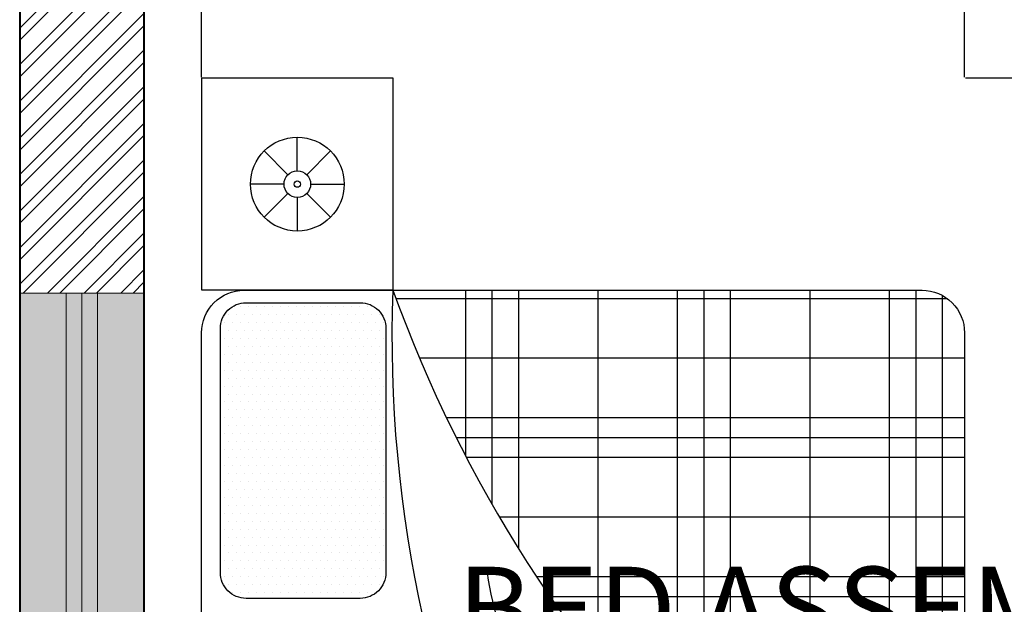
# Model space of a CAD drawing. Units: inches. Extents: x 528 to 2520, y -151 to 1354.
# Tile 5 of 41: x 587 to 658, y 1189 to 1232. Entities that reach past the tile are written whole.
import ezdxf

# ---------------------------------------------------------------- set-up
doc = ezdxf.new("R2010")
doc.units = ezdxf.units.IN
doc.header["$MEASUREMENT"] = 0
for name, color, linetype, lineweight in [('A-ANNO-DIMS', 2, 'Continuous', 18), ('A-FURN', 8, 'Continuous', 18), ('A-WALL-PATT', 6, 'Continuous', 13), ('walls', 7, 'Continuous', 40), ('WINDOWS', 2, 'Continuous', 20)]:
    doc.layers.add(name, color=color, linetype=linetype, lineweight=lineweight)
doc.layers.add('A-GLAZ-PATT', color=152, linetype='Continuous', lineweight=13, true_color=0x2776bb)
doc.layers.add('BLOCK', color=6, linetype='Continuous')
doc.styles.get("Standard").update_dxf_attribs({"font": 'arial.ttf'})
doc.dimstyles.get("Standard").update_dxf_attribs({"dimtxt": 6, "dimasz": 2, "dimexe": 0.18, "dimexo": 0.0625, "dimgap": 0.09, "dimtad": 0, "dimtih": 1, "dimtoh": 1, "dimdec": 1, "dimzin": 0, "dimdsep": 46, "dimlunit": 3, "dimtxsty": 'Standard', "dimblk": 'ARCHTICK', "dimcen": 0.09, "dimadec": 0, "dimazin": 0, "dimtfac": 1, "dimtdec": 1, "dimtofl": 0, "dimtmove": 0, "dimatfit": 3, "dimfxl": 1, "dimtolj": 1, "dimtzin": 0, "dimarcsym": 0})

# ---------------------------------------------------------------- blocks, each defined once
blk = doc.blocks.new('*X15')
at = {"color": 0}
for p, q in [((276.598, 451.25), (280.51, 451.25)), ((275.455, 450.625), (280.51, 450.625)), ((274.411, 450), (280.51, 450)), ((265.51, 448.125), (267.634, 448.125)), ((271.723, 448.125), (280.51, 448.125)), ((265.51, 446.25), (268.465, 446.25)), ((269.519, 446.25), (280.51, 446.25)), ((265.51, 445.625), (268.531, 445.625)), ((268.866, 445.625), (280.51, 445.625)), ((265.51, 445), (280.51, 445)), ((265.51, 443.125), (280.51, 443.125)), ((265.51, 441.25), (280.51, 441.25)), ((265.51, 440.625), (280.51, 440.625)), ((265.634, 440), (280.386, 440))]:
    blk.add_line(p, q, dxfattribs=at)
blk = doc.blocks.new('*X16')
at = {"color": 0}
for p, q in [((280.312, 439.886), (280.312, 452.896)), ((278.906, 439.482), (278.906, 452.338)), ((277.5, 439.482), (277.5, 451.702)), ((277.031, 439.482), (277.031, 451.471)), ((276.562, 439.482), (276.562, 451.231)), ((275.156, 439.482), (275.156, 450.451)), ((265.781, 439.797), (265.781, 449.511)), ((273.75, 439.482), (273.75, 449.576)), ((266.25, 439.517), (266.25, 449.296)), ((273.281, 439.482), (273.281, 449.261)), ((272.812, 439.482), (272.812, 448.934)), ((267.656, 439.482), (267.656, 448.095)), ((271.406, 439.482), (271.406, 447.876)), ((270, 439.482), (270, 446.689)), ((269.531, 439.482), (269.531, 446.262)), ((269.062, 439.482), (269.062, 445.817))]:
    blk.add_line(p, q, dxfattribs=at)
blk = doc.blocks.new('*X17')
at = {"color": 0}
for p, q in [((273.9375, 457.03125), (273.9375, 457.03125)), ((274.3125, 457.03125), (274.3125, 457.03125)), ((274.6875, 457.03125), (274.6875, 457.03125)), ((275.0625, 457.03125), (275.0625, 457.03125)), ((275.4375, 457.03125), (275.4375, 457.03125)), ((275.8125, 457.03125), (275.8125, 457.03125)), ((276.1875, 457.03125), (276.1875, 457.03125)), ((276.5625, 457.03125), (276.5625, 457.03125)), ((276.9375, 457.03125), (276.9375, 457.03125)), ((277.3125, 457.03125), (277.3125, 457.03125)), ((277.6875, 457.03125), (277.6875, 457.03125)), ((278.0625, 457.03125), (278.0625, 457.03125)), ((278.4375, 457.03125), (278.4375, 457.03125)), ((278.8125, 457.03125), (278.8125, 457.03125)), ((279.1875, 457.03125), (279.1875, 457.03125)), ((279.5625, 457.03125), (279.5625, 457.03125)), ((273.375, 456.75), (273.375, 456.75)), ((273.5625, 456.84375), (273.5625, 456.84375)), ((273.75, 456.9375), (273.75, 456.9375)), ((273.75, 456.75), (273.75, 456.75)), ((273.9375, 456.84375), (273.9375, 456.84375)), ((274.125, 456.9375), (274.125, 456.9375)), ((274.125, 456.75), (274.125, 456.75)), ((274.3125, 456.84375), (274.3125, 456.84375)), ((274.5, 456.9375), (274.5, 456.9375)), ((274.5, 456.75), (274.5, 456.75)), ((274.6875, 456.84375), (274.6875, 456.84375)), ((274.875, 456.9375), (274.875, 456.9375)), ((274.875, 456.75), (274.875, 456.75)), ((275.0625, 456.84375), (275.0625, 456.84375)), ((275.25, 456.9375), (275.25, 456.9375)), ((275.25, 456.75), (275.25, 456.75)), ((275.4375, 456.84375), (275.4375, 456.84375)), ((275.625, 456.9375), (275.625, 456.9375)), ((275.625, 456.75), (275.625, 456.75)), ((275.8125, 456.84375), (275.8125, 456.84375)), ((276, 456.9375), (276, 456.9375)), ((276, 456.75), (276, 456.75)), ((276.1875, 456.84375), (276.1875, 456.84375)), ((276.375, 456.9375), (276.375, 456.9375)), ((276.375, 456.75), (276.375, 456.75)), ((276.5625, 456.84375), (276.5625, 456.84375)), ((276.75, 456.9375), (276.75, 456.9375)), ((276.75, 456.75), (276.75, 456.75)), ((276.9375, 456.84375), (276.9375, 456.84375)), ((277.125, 456.9375), (277.125, 456.9375)), ((277.125, 456.75), (277.125, 456.75)), ((277.3125, 456.84375), (277.3125, 456.84375)), ((277.5, 456.9375), (277.5, 456.9375)), ((277.5, 456.75), (277.5, 456.75)), ((277.6875, 456.84375), (277.6875, 456.84375)), ((277.875, 456.9375), (277.875, 456.9375)), ((277.875, 456.75), (277.875, 456.75)), ((278.0625, 456.84375), (278.0625, 456.84375)), ((278.25, 456.9375), (278.25, 456.9375)), ((278.25, 456.75), (278.25, 456.75)), ((278.4375, 456.84375), (278.4375, 456.84375)), ((278.625, 456.9375), (278.625, 456.9375)), ((278.625, 456.75), (278.625, 456.75)), ((278.8125, 456.84375), (278.8125, 456.84375)), ((279, 456.9375), (279, 456.9375)), ((279, 456.75), (279, 456.75)), ((279.1875, 456.84375), (279.1875, 456.84375)), ((279.375, 456.9375), (279.375, 456.9375)), ((279.375, 456.75), (279.375, 456.75)), ((279.5625, 456.84375), (279.5625, 456.84375)), ((279.75, 456.9375), (279.75, 456.9375)), ((279.75, 456.75), (279.75, 456.75)), ((279.9375, 456.84375), (279.9375, 456.84375)), ((280.125, 456.75), (280.125, 456.75)), ((273.375, 456.5625), (273.375, 456.5625)), ((273.5625, 456.65625), (273.5625, 456.65625)), ((273.75, 456.5625), (273.75, 456.5625)), ((273.9375, 456.65625), (273.9375, 456.65625)), ((274.125, 456.5625), (274.125, 456.5625)), ((274.3125, 456.65625), (274.3125, 456.65625)), ((274.5, 456.5625), (274.5, 456.5625)), ((274.6875, 456.65625), (274.6875, 456.65625)), ((274.875, 456.5625), (274.875, 456.5625)), ((275.0625, 456.65625), (275.0625, 456.65625)), ((275.25, 456.5625), (275.25, 456.5625)), ((275.4375, 456.65625), (275.4375, 456.65625)), ((275.625, 456.5625), (275.625, 456.5625)), ((275.8125, 456.65625), (275.8125, 456.65625)), ((276, 456.5625), (276, 456.5625)), ((276.1875, 456.65625), (276.1875, 456.65625)), ((276.375, 456.5625), (276.375, 456.5625)), ((276.5625, 456.65625), (276.5625, 456.65625)), ((276.75, 456.5625), (276.75, 456.5625)), ((276.9375, 456.65625), (276.9375, 456.65625)), ((277.125, 456.5625), (277.125, 456.5625)), ((277.3125, 456.65625), (277.3125, 456.65625)), ((277.5, 456.5625), (277.5, 456.5625)), ((277.6875, 456.65625), (277.6875, 456.65625)), ((277.875, 456.5625), (277.875, 456.5625)), ((278.0625, 456.65625), (278.0625, 456.65625)), ((278.25, 456.5625), (278.25, 456.5625)), ((278.4375, 456.65625), (278.4375, 456.65625)), ((278.625, 456.5625), (278.625, 456.5625)), ((278.8125, 456.65625), (278.8125, 456.65625)), ((279, 456.5625), (279, 456.5625)), ((279.1875, 456.65625), (279.1875, 456.65625)), ((279.375, 456.5625), (279.375, 456.5625)), ((279.5625, 456.65625), (279.5625, 456.65625)), ((279.75, 456.5625), (279.75, 456.5625)), ((279.9375, 456.65625), (279.9375, 456.65625)), ((280.125, 456.5625), (280.125, 456.5625)), ((273.375, 456.375), (273.375, 456.375)), ((273.5625, 456.46875), (273.5625, 456.46875)), ((273.5625, 456.28125), (273.5625, 456.28125)), ((273.75, 456.375), (273.75, 456.375)), ((273.9375, 456.46875), (273.9375, 456.46875)), ((273.9375, 456.28125), (273.9375, 456.28125)), ((274.125, 456.375), (274.125, 456.375)), ((274.3125, 456.46875), (274.3125, 456.46875)), ((274.3125, 456.28125), (274.3125, 456.28125)), ((274.5, 456.375), (274.5, 456.375)), ((274.6875, 456.46875), (274.6875, 456.46875)), ((274.6875, 456.28125), (274.6875, 456.28125)), ((274.875, 456.375), (274.875, 456.375)), ((275.0625, 456.46875), (275.0625, 456.46875)), ((275.0625, 456.28125), (275.0625, 456.28125)), ((275.25, 456.375), (275.25, 456.375)), ((275.4375, 456.46875), (275.4375, 456.46875)), ((275.4375, 456.28125), (275.4375, 456.28125)), ((275.625, 456.375), (275.625, 456.375)), ((275.8125, 456.46875), (275.8125, 456.46875)), ((275.8125, 456.28125), (275.8125, 456.28125)), ((276, 456.375), (276, 456.375)), ((276.1875, 456.46875), (276.1875, 456.46875)), ((276.1875, 456.28125), (276.1875, 456.28125)), ((276.375, 456.375), (276.375, 456.375)), ((276.5625, 456.46875), (276.5625, 456.46875)), ((276.5625, 456.28125), (276.5625, 456.28125)), ((276.75, 456.375), (276.75, 456.375)), ((276.9375, 456.46875), (276.9375, 456.46875)), ((276.9375, 456.28125), (276.9375, 456.28125)), ((277.125, 456.375), (277.125, 456.375)), ((277.3125, 456.46875), (277.3125, 456.46875)), ((277.3125, 456.28125), (277.3125, 456.28125)), ((277.5, 456.375), (277.5, 456.375)), ((277.6875, 456.46875), (277.6875, 456.46875)), ((277.6875, 456.28125), (277.6875, 456.28125)), ((277.875, 456.375), (277.875, 456.375)), ((278.0625, 456.46875), (278.0625, 456.46875)), ((278.0625, 456.28125), (278.0625, 456.28125)), ((278.25, 456.375), (278.25, 456.375)), ((278.4375, 456.46875), (278.4375, 456.46875)), ((278.4375, 456.28125), (278.4375, 456.28125)), ((278.625, 456.375), (278.625, 456.375)), ((278.8125, 456.46875), (278.8125, 456.46875)), ((278.8125, 456.28125), (278.8125, 456.28125)), ((279, 456.375), (279, 456.375)), ((279.1875, 456.46875), (279.1875, 456.46875)), ((279.1875, 456.28125), (279.1875, 456.28125)), ((279.375, 456.375), (279.375, 456.375)), ((279.5625, 456.46875), (279.5625, 456.46875)), ((279.5625, 456.28125), (279.5625, 456.28125)), ((279.75, 456.375), (279.75, 456.375)), ((279.9375, 456.46875), (279.9375, 456.46875)), ((279.9375, 456.28125), (279.9375, 456.28125)), ((280.125, 456.375), (280.125, 456.375)), ((273.375, 456.1875), (273.375, 456.1875)), ((273.5625, 456.09375), (273.5625, 456.09375)), ((273.75, 456.1875), (273.75, 456.1875)), ((273.9375, 456.09375), (273.9375, 456.09375)), ((274.125, 456.1875), (274.125, 456.1875)), ((274.3125, 456.09375), (274.3125, 456.09375)), ((274.5, 456.1875), (274.5, 456.1875)), ((274.6875, 456.09375), (274.6875, 456.09375)), ((274.875, 456.1875), (274.875, 456.1875)), ((275.0625, 456.09375), (275.0625, 456.09375)), ((275.25, 456.1875), (275.25, 456.1875)), ((275.4375, 456.09375), (275.4375, 456.09375)), ((275.625, 456.1875), (275.625, 456.1875)), ((275.8125, 456.09375), (275.8125, 456.09375)), ((276, 456.1875), (276, 456.1875)), ((276.1875, 456.09375), (276.1875, 456.09375)), ((276.375, 456.1875), (276.375, 456.1875)), ((276.5625, 456.09375), (276.5625, 456.09375)), ((276.75, 456.1875), (276.75, 456.1875)), ((276.9375, 456.09375), (276.9375, 456.09375)), ((277.125, 456.1875), (277.125, 456.1875)), ((277.3125, 456.09375), (277.3125, 456.09375)), ((277.5, 456.1875), (277.5, 456.1875)), ((277.6875, 456.09375), (277.6875, 456.09375)), ((277.875, 456.1875), (277.875, 456.1875)), ((278.0625, 456.09375), (278.0625, 456.09375)), ((278.25, 456.1875), (278.25, 456.1875)), ((278.4375, 456.09375), (278.4375, 456.09375)), ((278.625, 456.1875), (278.625, 456.1875)), ((278.8125, 456.09375), (278.8125, 456.09375)), ((279, 456.1875), (279, 456.1875)), ((279.1875, 456.09375), (279.1875, 456.09375)), ((279.375, 456.1875), (279.375, 456.1875)), ((279.5625, 456.09375), (279.5625, 456.09375)), ((279.75, 456.1875), (279.75, 456.1875)), ((279.9375, 456.09375), (279.9375, 456.09375)), ((280.125, 456.1875), (280.125, 456.1875)), ((273.375, 456), (273.375, 456)), ((273.375, 455.8125), (273.375, 455.8125)), ((273.5625, 455.90625), (273.5625, 455.90625)), ((273.75, 456), (273.75, 456)), ((273.75, 455.8125), (273.75, 455.8125)), ((273.9375, 455.90625), (273.9375, 455.90625)), ((274.125, 456), (274.125, 456)), ((274.125, 455.8125), (274.125, 455.8125)), ((274.3125, 455.90625), (274.3125, 455.90625)), ((274.5, 456), (274.5, 456)), ((274.5, 455.8125), (274.5, 455.8125)), ((274.6875, 455.90625), (274.6875, 455.90625)), ((274.875, 456), (274.875, 456)), ((274.875, 455.8125), (274.875, 455.8125)), ((275.0625, 455.90625), (275.0625, 455.90625)), ((275.25, 456), (275.25, 456)), ((275.25, 455.8125), (275.25, 455.8125)), ((275.4375, 455.90625), (275.4375, 455.90625)), ((275.625, 456), (275.625, 456)), ((275.625, 455.8125), (275.625, 455.8125)), ((275.8125, 455.90625), (275.8125, 455.90625)), ((276, 456), (276, 456)), ((276, 455.8125), (276, 455.8125)), ((276.1875, 455.90625), (276.1875, 455.90625)), ((276.375, 456), (276.375, 456)), ((276.375, 455.8125), (276.375, 455.8125)), ((276.5625, 455.90625), (276.5625, 455.90625)), ((276.75, 456), (276.75, 456)), ((276.75, 455.8125), (276.75, 455.8125)), ((276.9375, 455.90625), (276.9375, 455.90625)), ((277.125, 456), (277.125, 456)), ((277.125, 455.8125), (277.125, 455.8125)), ((277.3125, 455.90625), (277.3125, 455.90625)), ((277.5, 456), (277.5, 456)), ((277.5, 455.8125), (277.5, 455.8125)), ((277.6875, 455.90625), (277.6875, 455.90625)), ((277.875, 456), (277.875, 456)), ((277.875, 455.8125), (277.875, 455.8125)), ((278.0625, 455.90625), (278.0625, 455.90625)), ((278.25, 456), (278.25, 456)), ((278.25, 455.8125), (278.25, 455.8125)), ((278.4375, 455.90625), (278.4375, 455.90625)), ((278.625, 456), (278.625, 456)), ((278.625, 455.8125), (278.625, 455.8125)), ((278.8125, 455.90625), (278.8125, 455.90625)), ((279, 456), (279, 456)), ((279, 455.8125), (279, 455.8125)), ((279.1875, 455.90625), (279.1875, 455.90625)), ((279.375, 456), (279.375, 456)), ((279.375, 455.8125), (279.375, 455.8125)), ((279.5625, 455.90625), (279.5625, 455.90625)), ((279.75, 456), (279.75, 456)), ((279.75, 455.8125), (279.75, 455.8125)), ((279.9375, 455.90625), (279.9375, 455.90625)), ((280.125, 456), (280.125, 456)), ((280.125, 455.8125), (280.125, 455.8125)), ((273.375, 455.625), (273.375, 455.625)), ((273.5625, 455.71875), (273.5625, 455.71875)), ((273.75, 455.625), (273.75, 455.625)), ((273.9375, 455.71875), (273.9375, 455.71875)), ((274.125, 455.625), (274.125, 455.625)), ((274.3125, 455.71875), (274.3125, 455.71875)), ((274.5, 455.625), (274.5, 455.625)), ((274.6875, 455.71875), (274.6875, 455.71875)), ((274.875, 455.625), (274.875, 455.625)), ((275.0625, 455.71875), (275.0625, 455.71875)), ((275.25, 455.625), (275.25, 455.625)), ((275.4375, 455.71875), (275.4375, 455.71875)), ((275.625, 455.625), (275.625, 455.625)), ((275.8125, 455.71875), (275.8125, 455.71875)), ((276, 455.625), (276, 455.625)), ((276.1875, 455.71875), (276.1875, 455.71875)), ((276.375, 455.625), (276.375, 455.625)), ((276.5625, 455.71875), (276.5625, 455.71875)), ((276.75, 455.625), (276.75, 455.625)), ((276.9375, 455.71875), (276.9375, 455.71875)), ((277.125, 455.625), (277.125, 455.625)), ((277.3125, 455.71875), (277.3125, 455.71875)), ((277.5, 455.625), (277.5, 455.625)), ((277.6875, 455.71875), (277.6875, 455.71875)), ((277.875, 455.625), (277.875, 455.625)), ((278.0625, 455.71875), (278.0625, 455.71875)), ((278.25, 455.625), (278.25, 455.625)), ((278.4375, 455.71875), (278.4375, 455.71875)), ((278.625, 455.625), (278.625, 455.625)), ((278.8125, 455.71875), (278.8125, 455.71875)), ((279, 455.625), (279, 455.625)), ((279.1875, 455.71875), (279.1875, 455.71875)), ((279.375, 455.625), (279.375, 455.625)), ((279.5625, 455.71875), (279.5625, 455.71875)), ((279.75, 455.625), (279.75, 455.625)), ((279.9375, 455.71875), (279.9375, 455.71875)), ((280.125, 455.625), (280.125, 455.625)), ((273.375, 455.4375), (273.375, 455.4375)), ((273.5625, 455.53125), (273.5625, 455.53125)), ((273.5625, 455.34375), (273.5625, 455.34375)), ((273.75, 455.4375), (273.75, 455.4375)), ((273.9375, 455.53125), (273.9375, 455.53125)), ((273.9375, 455.34375), (273.9375, 455.34375)), ((274.125, 455.4375), (274.125, 455.4375)), ((274.3125, 455.53125), (274.3125, 455.53125)), ((274.3125, 455.34375), (274.3125, 455.34375)), ((274.5, 455.4375), (274.5, 455.4375)), ((274.6875, 455.53125), (274.6875, 455.53125)), ((274.6875, 455.34375), (274.6875, 455.34375)), ((274.875, 455.4375), (274.875, 455.4375)), ((275.0625, 455.53125), (275.0625, 455.53125)), ((275.0625, 455.34375), (275.0625, 455.34375)), ((275.25, 455.4375), (275.25, 455.4375)), ((275.4375, 455.53125), (275.4375, 455.53125)), ((275.4375, 455.34375), (275.4375, 455.34375)), ((275.625, 455.4375), (275.625, 455.4375)), ((275.8125, 455.53125), (275.8125, 455.53125)), ((275.8125, 455.34375), (275.8125, 455.34375)), ((276, 455.4375), (276, 455.4375)), ((276.1875, 455.53125), (276.1875, 455.53125)), ((276.1875, 455.34375), (276.1875, 455.34375)), ((276.375, 455.4375), (276.375, 455.4375)), ((276.5625, 455.53125), (276.5625, 455.53125)), ((276.5625, 455.34375), (276.5625, 455.34375)), ((276.75, 455.4375), (276.75, 455.4375)), ((276.9375, 455.53125), (276.9375, 455.53125)), ((276.9375, 455.34375), (276.9375, 455.34375)), ((277.125, 455.4375), (277.125, 455.4375)), ((277.3125, 455.53125), (277.3125, 455.53125)), ((277.3125, 455.34375), (277.3125, 455.34375)), ((277.5, 455.4375), (277.5, 455.4375)), ((277.6875, 455.53125), (277.6875, 455.53125)), ((277.6875, 455.34375), (277.6875, 455.34375)), ((277.875, 455.4375), (277.875, 455.4375)), ((278.0625, 455.53125), (278.0625, 455.53125)), ((278.0625, 455.34375), (278.0625, 455.34375)), ((278.25, 455.4375), (278.25, 455.4375)), ((278.4375, 455.53125), (278.4375, 455.53125)), ((278.4375, 455.34375), (278.4375, 455.34375)), ((278.625, 455.4375), (278.625, 455.4375)), ((278.8125, 455.53125), (278.8125, 455.53125)), ((278.8125, 455.34375), (278.8125, 455.34375)), ((279, 455.4375), (279, 455.4375)), ((279.1875, 455.53125), (279.1875, 455.53125)), ((279.1875, 455.34375), (279.1875, 455.34375)), ((279.375, 455.4375), (279.375, 455.4375)), ((279.5625, 455.53125), (279.5625, 455.53125)), ((279.5625, 455.34375), (279.5625, 455.34375)), ((279.75, 455.4375), (279.75, 455.4375)), ((279.9375, 455.53125), (279.9375, 455.53125)), ((279.9375, 455.34375), (279.9375, 455.34375)), ((280.125, 455.4375), (280.125, 455.4375)), ((273.375, 455.25), (273.375, 455.25)), ((273.5625, 455.15625), (273.5625, 455.15625)), ((273.75, 455.25), (273.75, 455.25)), ((273.9375, 455.15625), (273.9375, 455.15625)), ((274.125, 455.25), (274.125, 455.25)), ((274.3125, 455.15625), (274.3125, 455.15625)), ((274.5, 455.25), (274.5, 455.25)), ((274.6875, 455.15625), (274.6875, 455.15625)), ((274.875, 455.25), (274.875, 455.25)), ((275.0625, 455.15625), (275.0625, 455.15625)), ((275.25, 455.25), (275.25, 455.25)), ((275.4375, 455.15625), (275.4375, 455.15625)), ((275.625, 455.25), (275.625, 455.25)), ((275.8125, 455.15625), (275.8125, 455.15625)), ((276, 455.25), (276, 455.25)), ((276.1875, 455.15625), (276.1875, 455.15625)), ((276.375, 455.25), (276.375, 455.25)), ((276.5625, 455.15625), (276.5625, 455.15625)), ((276.75, 455.25), (276.75, 455.25)), ((276.9375, 455.15625), (276.9375, 455.15625)), ((277.125, 455.25), (277.125, 455.25)), ((277.3125, 455.15625), (277.3125, 455.15625)), ((277.5, 455.25), (277.5, 455.25)), ((277.6875, 455.15625), (277.6875, 455.15625)), ((277.875, 455.25), (277.875, 455.25)), ((278.0625, 455.15625), (278.0625, 455.15625)), ((278.25, 455.25), (278.25, 455.25)), ((278.4375, 455.15625), (278.4375, 455.15625)), ((278.625, 455.25), (278.625, 455.25)), ((278.8125, 455.15625), (278.8125, 455.15625)), ((279, 455.25), (279, 455.25)), ((279.1875, 455.15625), (279.1875, 455.15625)), ((279.375, 455.25), (279.375, 455.25)), ((279.5625, 455.15625), (279.5625, 455.15625)), ((279.75, 455.25), (279.75, 455.25)), ((279.9375, 455.15625), (279.9375, 455.15625)), ((280.125, 455.25), (280.125, 455.25)), ((273.375, 455.0625), (273.375, 455.0625)), ((273.375, 454.875), (273.375, 454.875)), ((273.5625, 454.96875), (273.5625, 454.96875)), ((273.75, 455.0625), (273.75, 455.0625)), ((273.75, 454.875), (273.75, 454.875)), ((273.9375, 454.96875), (273.9375, 454.96875)), ((274.125, 455.0625), (274.125, 455.0625)), ((274.125, 454.875), (274.125, 454.875)), ((274.3125, 454.96875), (274.3125, 454.96875)), ((274.5, 455.0625), (274.5, 455.0625)), ((274.5, 454.875), (274.5, 454.875)), ((274.6875, 454.96875), (274.6875, 454.96875)), ((274.875, 455.0625), (274.875, 455.0625)), ((274.875, 454.875), (274.875, 454.875)), ((275.0625, 454.96875), (275.0625, 454.96875)), ((275.25, 455.0625), (275.25, 455.0625)), ((275.25, 454.875), (275.25, 454.875)), ((275.4375, 454.96875), (275.4375, 454.96875)), ((275.625, 455.0625), (275.625, 455.0625)), ((275.625, 454.875), (275.625, 454.875)), ((275.8125, 454.96875), (275.8125, 454.96875)), ((276, 455.0625), (276, 455.0625)), ((276, 454.875), (276, 454.875)), ((276.1875, 454.96875), (276.1875, 454.96875)), ((276.375, 455.0625), (276.375, 455.0625)), ((276.375, 454.875), (276.375, 454.875)), ((276.5625, 454.96875), (276.5625, 454.96875)), ((276.75, 455.0625), (276.75, 455.0625)), ((276.75, 454.875), (276.75, 454.875)), ((276.9375, 454.96875), (276.9375, 454.96875)), ((277.125, 455.0625), (277.125, 455.0625)), ((277.125, 454.875), (277.125, 454.875)), ((277.3125, 454.96875), (277.3125, 454.96875)), ((277.5, 455.0625), (277.5, 455.0625)), ((277.5, 454.875), (277.5, 454.875)), ((277.6875, 454.96875), (277.6875, 454.96875)), ((277.875, 455.0625), (277.875, 455.0625)), ((277.875, 454.875), (277.875, 454.875)), ((278.0625, 454.96875), (278.0625, 454.96875)), ((278.25, 455.0625), (278.25, 455.0625)), ((278.25, 454.875), (278.25, 454.875)), ((278.4375, 454.96875), (278.4375, 454.96875)), ((278.625, 455.0625), (278.625, 455.0625)), ((278.625, 454.875), (278.625, 454.875)), ((278.8125, 454.96875), (278.8125, 454.96875)), ((279, 455.0625), (279, 455.0625)), ((279, 454.875), (279, 454.875)), ((279.1875, 454.96875), (279.1875, 454.96875)), ((279.375, 455.0625), (279.375, 455.0625)), ((279.375, 454.875), (279.375, 454.875)), ((279.5625, 454.96875), (279.5625, 454.96875)), ((279.75, 455.0625), (279.75, 455.0625)), ((279.75, 454.875), (279.75, 454.875)), ((279.9375, 454.96875), (279.9375, 454.96875)), ((280.125, 455.0625), (280.125, 455.0625)), ((280.125, 454.875), (280.125, 454.875)), ((273.375, 454.6875), (273.375, 454.6875)), ((273.5625, 454.78125), (273.5625, 454.78125)), ((273.75, 454.6875), (273.75, 454.6875)), ((273.9375, 454.78125), (273.9375, 454.78125)), ((274.125, 454.6875), (274.125, 454.6875)), ((274.3125, 454.78125), (274.3125, 454.78125)), ((274.5, 454.6875), (274.5, 454.6875)), ((274.6875, 454.78125), (274.6875, 454.78125)), ((274.875, 454.6875), (274.875, 454.6875)), ((275.0625, 454.78125), (275.0625, 454.78125)), ((275.25, 454.6875), (275.25, 454.6875)), ((275.4375, 454.78125), (275.4375, 454.78125)), ((275.625, 454.6875), (275.625, 454.6875)), ((275.8125, 454.78125), (275.8125, 454.78125)), ((276, 454.6875), (276, 454.6875)), ((276.1875, 454.78125), (276.1875, 454.78125)), ((276.375, 454.6875), (276.375, 454.6875)), ((276.5625, 454.78125), (276.5625, 454.78125)), ((276.75, 454.6875), (276.75, 454.6875)), ((276.9375, 454.78125), (276.9375, 454.78125)), ((277.125, 454.6875), (277.125, 454.6875)), ((277.3125, 454.78125), (277.3125, 454.78125)), ((277.5, 454.6875), (277.5, 454.6875)), ((277.6875, 454.78125), (277.6875, 454.78125)), ((277.875, 454.6875), (277.875, 454.6875)), ((278.0625, 454.78125), (278.0625, 454.78125)), ((278.25, 454.6875), (278.25, 454.6875)), ((278.4375, 454.78125), (278.4375, 454.78125)), ((278.625, 454.6875), (278.625, 454.6875)), ((278.8125, 454.78125), (278.8125, 454.78125)), ((279, 454.6875), (279, 454.6875)), ((279.1875, 454.78125), (279.1875, 454.78125)), ((279.375, 454.6875), (279.375, 454.6875)), ((279.5625, 454.78125), (279.5625, 454.78125)), ((279.75, 454.6875), (279.75, 454.6875)), ((279.9375, 454.78125), (279.9375, 454.78125)), ((280.125, 454.6875), (280.125, 454.6875)), ((273.375, 454.5), (273.375, 454.5)), ((273.5625, 454.59375), (273.5625, 454.59375)), ((273.5625, 454.40625), (273.5625, 454.40625)), ((273.75, 454.5), (273.75, 454.5)), ((273.9375, 454.59375), (273.9375, 454.59375)), ((273.9375, 454.40625), (273.9375, 454.40625)), ((274.125, 454.5), (274.125, 454.5)), ((274.3125, 454.59375), (274.3125, 454.59375)), ((274.3125, 454.40625), (274.3125, 454.40625)), ((274.5, 454.5), (274.5, 454.5)), ((274.6875, 454.59375), (274.6875, 454.59375)), ((274.6875, 454.40625), (274.6875, 454.40625)), ((274.875, 454.5), (274.875, 454.5)), ((275.0625, 454.59375), (275.0625, 454.59375)), ((275.0625, 454.40625), (275.0625, 454.40625)), ((275.25, 454.5), (275.25, 454.5)), ((275.4375, 454.59375), (275.4375, 454.59375)), ((275.4375, 454.40625), (275.4375, 454.40625)), ((275.625, 454.5), (275.625, 454.5)), ((275.8125, 454.59375), (275.8125, 454.59375)), ((275.8125, 454.40625), (275.8125, 454.40625)), ((276, 454.5), (276, 454.5)), ((276.1875, 454.59375), (276.1875, 454.59375)), ((276.1875, 454.40625), (276.1875, 454.40625)), ((276.375, 454.5), (276.375, 454.5)), ((276.5625, 454.59375), (276.5625, 454.59375)), ((276.5625, 454.40625), (276.5625, 454.40625)), ((276.75, 454.5), (276.75, 454.5)), ((276.9375, 454.59375), (276.9375, 454.59375)), ((276.9375, 454.40625), (276.9375, 454.40625)), ((277.125, 454.5), (277.125, 454.5)), ((277.3125, 454.59375), (277.3125, 454.59375)), ((277.3125, 454.40625), (277.3125, 454.40625)), ((277.5, 454.5), (277.5, 454.5)), ((277.6875, 454.59375), (277.6875, 454.59375)), ((277.6875, 454.40625), (277.6875, 454.40625)), ((277.875, 454.5), (277.875, 454.5)), ((278.0625, 454.59375), (278.0625, 454.59375)), ((278.0625, 454.40625), (278.0625, 454.40625)), ((278.25, 454.5), (278.25, 454.5)), ((278.4375, 454.59375), (278.4375, 454.59375)), ((278.4375, 454.40625), (278.4375, 454.40625)), ((278.625, 454.5), (278.625, 454.5)), ((278.8125, 454.59375), (278.8125, 454.59375)), ((278.8125, 454.40625), (278.8125, 454.40625)), ((279, 454.5), (279, 454.5)), ((279.1875, 454.59375), (279.1875, 454.59375)), ((279.1875, 454.40625), (279.1875, 454.40625)), ((279.375, 454.5), (279.375, 454.5)), ((279.5625, 454.59375), (279.5625, 454.59375)), ((279.5625, 454.40625), (279.5625, 454.40625)), ((279.75, 454.5), (279.75, 454.5)), ((279.9375, 454.59375), (279.9375, 454.59375)), ((279.9375, 454.40625), (279.9375, 454.40625)), ((280.125, 454.5), (280.125, 454.5)), ((273.375, 454.3125), (273.375, 454.3125)), ((273.5625, 454.21875), (273.5625, 454.21875)), ((273.75, 454.3125), (273.75, 454.3125)), ((273.9375, 454.21875), (273.9375, 454.21875)), ((274.125, 454.3125), (274.125, 454.3125)), ((274.3125, 454.21875), (274.3125, 454.21875)), ((274.5, 454.3125), (274.5, 454.3125)), ((274.6875, 454.21875), (274.6875, 454.21875)), ((274.875, 454.3125), (274.875, 454.3125)), ((275.0625, 454.21875), (275.0625, 454.21875)), ((275.25, 454.3125), (275.25, 454.3125)), ((275.4375, 454.21875), (275.4375, 454.21875)), ((275.625, 454.3125), (275.625, 454.3125)), ((275.8125, 454.21875), (275.8125, 454.21875)), ((276, 454.3125), (276, 454.3125)), ((276.1875, 454.21875), (276.1875, 454.21875)), ((276.375, 454.3125), (276.375, 454.3125)), ((276.5625, 454.21875), (276.5625, 454.21875)), ((276.75, 454.3125), (276.75, 454.3125)), ((276.9375, 454.21875), (276.9375, 454.21875)), ((277.125, 454.3125), (277.125, 454.3125)), ((277.3125, 454.21875), (277.3125, 454.21875)), ((277.5, 454.3125), (277.5, 454.3125)), ((277.6875, 454.21875), (277.6875, 454.21875)), ((277.875, 454.3125), (277.875, 454.3125)), ((278.0625, 454.21875), (278.0625, 454.21875)), ((278.25, 454.3125), (278.25, 454.3125)), ((278.4375, 454.21875), (278.4375, 454.21875)), ((278.625, 454.3125), (278.625, 454.3125)), ((278.8125, 454.21875), (278.8125, 454.21875)), ((279, 454.3125), (279, 454.3125)), ((279.1875, 454.21875), (279.1875, 454.21875)), ((279.375, 454.3125), (279.375, 454.3125)), ((279.5625, 454.21875), (279.5625, 454.21875)), ((279.75, 454.3125), (279.75, 454.3125)), ((279.9375, 454.21875), (279.9375, 454.21875)), ((280.125, 454.3125), (280.125, 454.3125)), ((273.375, 454.125), (273.375, 454.125)), ((273.375, 453.9375), (273.375, 453.9375)), ((273.5625, 454.03125), (273.5625, 454.03125)), ((273.75, 454.125), (273.75, 454.125)), ((273.75, 453.9375), (273.75, 453.9375)), ((273.9375, 454.03125), (273.9375, 454.03125)), ((274.125, 454.125), (274.125, 454.125)), ((274.125, 453.9375), (274.125, 453.9375)), ((274.3125, 454.03125), (274.3125, 454.03125)), ((274.5, 454.125), (274.5, 454.125)), ((274.5, 453.9375), (274.5, 453.9375)), ((274.6875, 454.03125), (274.6875, 454.03125)), ((274.875, 454.125), (274.875, 454.125)), ((274.875, 453.9375), (274.875, 453.9375)), ((275.0625, 454.03125), (275.0625, 454.03125)), ((275.25, 454.125), (275.25, 454.125)), ((275.25, 453.9375), (275.25, 453.9375)), ((275.4375, 454.03125), (275.4375, 454.03125)), ((275.625, 454.125), (275.625, 454.125)), ((275.625, 453.9375), (275.625, 453.9375)), ((275.8125, 454.03125), (275.8125, 454.03125)), ((276, 454.125), (276, 454.125)), ((276, 453.9375), (276, 453.9375)), ((276.1875, 454.03125), (276.1875, 454.03125)), ((276.375, 454.125), (276.375, 454.125)), ((276.375, 453.9375), (276.375, 453.9375)), ((276.5625, 454.03125), (276.5625, 454.03125)), ((276.75, 454.125), (276.75, 454.125)), ((276.75, 453.9375), (276.75, 453.9375)), ((276.9375, 454.03125), (276.9375, 454.03125)), ((277.125, 454.125), (277.125, 454.125)), ((277.125, 453.9375), (277.125, 453.9375)), ((277.3125, 454.03125), (277.3125, 454.03125)), ((277.5, 454.125), (277.5, 454.125)), ((277.5, 453.9375), (277.5, 453.9375)), ((277.6875, 454.03125), (277.6875, 454.03125)), ((277.875, 454.125), (277.875, 454.125)), ((277.875, 453.9375), (277.875, 453.9375)), ((278.0625, 454.03125), (278.0625, 454.03125)), ((278.25, 454.125), (278.25, 454.125)), ((278.25, 453.9375), (278.25, 453.9375)), ((278.4375, 454.03125), (278.4375, 454.03125)), ((278.625, 454.125), (278.625, 454.125)), ((278.625, 453.9375), (278.625, 453.9375)), ((278.8125, 454.03125), (278.8125, 454.03125)), ((279, 454.125), (279, 454.125)), ((279, 453.9375), (279, 453.9375)), ((279.1875, 454.03125), (279.1875, 454.03125)), ((279.375, 454.125), (279.375, 454.125)), ((279.375, 453.9375), (279.375, 453.9375)), ((279.5625, 454.03125), (279.5625, 454.03125)), ((279.75, 454.125), (279.75, 454.125)), ((279.75, 453.9375), (279.75, 453.9375)), ((279.9375, 454.03125), (279.9375, 454.03125)), ((280.125, 454.125), (280.125, 454.125)), ((280.125, 453.9375), (280.125, 453.9375)), ((273.375, 453.75), (273.375, 453.75)), ((273.5625, 453.84375), (273.5625, 453.84375)), ((273.75, 453.75), (273.75, 453.75)), ((273.9375, 453.84375), (273.9375, 453.84375)), ((274.125, 453.75), (274.125, 453.75)), ((274.3125, 453.84375), (274.3125, 453.84375)), ((274.5, 453.75), (274.5, 453.75)), ((274.6875, 453.84375), (274.6875, 453.84375)), ((274.875, 453.75), (274.875, 453.75)), ((275.0625, 453.84375), (275.0625, 453.84375)), ((275.25, 453.75), (275.25, 453.75)), ((275.4375, 453.84375), (275.4375, 453.84375)), ((275.625, 453.75), (275.625, 453.75)), ((275.8125, 453.84375), (275.8125, 453.84375)), ((276, 453.75), (276, 453.75)), ((276.1875, 453.84375), (276.1875, 453.84375)), ((276.375, 453.75), (276.375, 453.75)), ((276.5625, 453.84375), (276.5625, 453.84375)), ((276.75, 453.75), (276.75, 453.75)), ((276.9375, 453.84375), (276.9375, 453.84375)), ((277.125, 453.75), (277.125, 453.75)), ((277.3125, 453.84375), (277.3125, 453.84375)), ((277.5, 453.75), (277.5, 453.75)), ((277.6875, 453.84375), (277.6875, 453.84375)), ((277.875, 453.75), (277.875, 453.75)), ((278.0625, 453.84375), (278.0625, 453.84375)), ((278.25, 453.75), (278.25, 453.75)), ((278.4375, 453.84375), (278.4375, 453.84375)), ((278.625, 453.75), (278.625, 453.75)), ((278.8125, 453.84375), (278.8125, 453.84375)), ((279, 453.75), (279, 453.75)), ((279.1875, 453.84375), (279.1875, 453.84375)), ((279.375, 453.75), (279.375, 453.75)), ((279.5625, 453.84375), (279.5625, 453.84375)), ((279.75, 453.75), (279.75, 453.75)), ((279.9375, 453.84375), (279.9375, 453.84375)), ((280.125, 453.75), (280.125, 453.75)), ((273.375, 453.5625), (273.375, 453.5625)), ((273.5625, 453.65625), (273.5625, 453.65625)), ((273.5625, 453.46875), (273.5625, 453.46875)), ((273.75, 453.5625), (273.75, 453.5625)), ((273.9375, 453.65625), (273.9375, 453.65625)), ((273.9375, 453.46875), (273.9375, 453.46875)), ((274.125, 453.5625), (274.125, 453.5625)), ((274.3125, 453.65625), (274.3125, 453.65625)), ((274.3125, 453.46875), (274.3125, 453.46875)), ((274.5, 453.5625), (274.5, 453.5625)), ((274.6875, 453.65625), (274.6875, 453.65625)), ((274.6875, 453.46875), (274.6875, 453.46875)), ((274.875, 453.5625), (274.875, 453.5625)), ((275.0625, 453.65625), (275.0625, 453.65625)), ((275.0625, 453.46875), (275.0625, 453.46875)), ((275.25, 453.5625), (275.25, 453.5625)), ((275.4375, 453.65625), (275.4375, 453.65625)), ((275.4375, 453.46875), (275.4375, 453.46875)), ((275.625, 453.5625), (275.625, 453.5625)), ((275.8125, 453.65625), (275.8125, 453.65625)), ((275.8125, 453.46875), (275.8125, 453.46875)), ((276, 453.5625), (276, 453.5625)), ((276.1875, 453.65625), (276.1875, 453.65625)), ((276.1875, 453.46875), (276.1875, 453.46875)), ((276.375, 453.5625), (276.375, 453.5625)), ((276.5625, 453.65625), (276.5625, 453.65625)), ((276.5625, 453.46875), (276.5625, 453.46875)), ((276.75, 453.5625), (276.75, 453.5625)), ((276.9375, 453.65625), (276.9375, 453.65625)), ((276.9375, 453.46875), (276.9375, 453.46875)), ((277.125, 453.5625), (277.125, 453.5625)), ((277.3125, 453.65625), (277.3125, 453.65625)), ((277.3125, 453.46875), (277.3125, 453.46875)), ((277.5, 453.5625), (277.5, 453.5625)), ((277.6875, 453.65625), (277.6875, 453.65625)), ((277.6875, 453.46875), (277.6875, 453.46875)), ((277.875, 453.5625), (277.875, 453.5625)), ((278.0625, 453.65625), (278.0625, 453.65625)), ((278.0625, 453.46875), (278.0625, 453.46875)), ((278.25, 453.5625), (278.25, 453.5625)), ((278.4375, 453.65625), (278.4375, 453.65625)), ((278.4375, 453.46875), (278.4375, 453.46875)), ((278.625, 453.5625), (278.625, 453.5625)), ((278.8125, 453.65625), (278.8125, 453.65625)), ((278.8125, 453.46875), (278.8125, 453.46875)), ((279, 453.5625), (279, 453.5625)), ((279.1875, 453.65625), (279.1875, 453.65625)), ((279.1875, 453.46875), (279.1875, 453.46875)), ((279.375, 453.5625), (279.375, 453.5625)), ((279.5625, 453.65625), (279.5625, 453.65625)), ((279.5625, 453.46875), (279.5625, 453.46875)), ((279.75, 453.5625), (279.75, 453.5625)), ((279.9375, 453.65625), (279.9375, 453.65625)), ((279.9375, 453.46875), (279.9375, 453.46875)), ((280.125, 453.5625), (280.125, 453.5625)), ((273.375, 453.375), (273.375, 453.375)), ((273.5625, 453.28125), (273.5625, 453.28125)), ((273.75, 453.375), (273.75, 453.375)), ((273.9375, 453.28125), (273.9375, 453.28125)), ((274.125, 453.375), (274.125, 453.375)), ((274.3125, 453.28125), (274.3125, 453.28125)), ((274.5, 453.375), (274.5, 453.375)), ((274.6875, 453.28125), (274.6875, 453.28125)), ((274.875, 453.375), (274.875, 453.375)), ((275.0625, 453.28125), (275.0625, 453.28125)), ((275.25, 453.375), (275.25, 453.375)), ((275.4375, 453.28125), (275.4375, 453.28125)), ((275.625, 453.375), (275.625, 453.375)), ((275.8125, 453.28125), (275.8125, 453.28125)), ((276, 453.375), (276, 453.375)), ((276.1875, 453.28125), (276.1875, 453.28125)), ((276.375, 453.375), (276.375, 453.375)), ((276.5625, 453.28125), (276.5625, 453.28125)), ((276.75, 453.375), (276.75, 453.375)), ((276.9375, 453.28125), (276.9375, 453.28125)), ((277.125, 453.375), (277.125, 453.375)), ((277.3125, 453.28125), (277.3125, 453.28125)), ((277.5, 453.375), (277.5, 453.375)), ((277.6875, 453.28125), (277.6875, 453.28125)), ((277.875, 453.375), (277.875, 453.375)), ((278.0625, 453.28125), (278.0625, 453.28125)), ((278.25, 453.375), (278.25, 453.375)), ((278.4375, 453.28125), (278.4375, 453.28125)), ((278.625, 453.375), (278.625, 453.375)), ((278.8125, 453.28125), (278.8125, 453.28125)), ((279, 453.375), (279, 453.375)), ((279.1875, 453.28125), (279.1875, 453.28125)), ((279.375, 453.375), (279.375, 453.375)), ((279.5625, 453.28125), (279.5625, 453.28125)), ((279.75, 453.375), (279.75, 453.375)), ((279.9375, 453.28125), (279.9375, 453.28125)), ((273.75, 453.1875), (273.75, 453.1875)), ((274.125, 453.1875), (274.125, 453.1875)), ((274.5, 453.1875), (274.5, 453.1875)), ((274.875, 453.1875), (274.875, 453.1875)), ((275.25, 453.1875), (275.25, 453.1875)), ((275.625, 453.1875), (275.625, 453.1875)), ((276, 453.1875), (276, 453.1875)), ((276.375, 453.1875), (276.375, 453.1875)), ((276.75, 453.1875), (276.75, 453.1875)), ((277.125, 453.1875), (277.125, 453.1875)), ((277.5, 453.1875), (277.5, 453.1875)), ((277.875, 453.1875), (277.875, 453.1875)), ((278.25, 453.1875), (278.25, 453.1875)), ((278.625, 453.1875), (278.625, 453.1875)), ((279, 453.1875), (279, 453.1875)), ((279.375, 453.1875), (279.375, 453.1875)), ((279.75, 453.1875), (279.75, 453.1875))]:
    blk.add_line(p, q, dxfattribs=at)
blk = doc.blocks.new('A$C52E67D0D')
at = {"layer": 'BLOCK'}
for p, q in [((2251.5, 1605.5), (2251.5, 1684.7)), ((2229.3, 1596.3), (2173.3, 1652.3)), ((2273.7, 1596.3), (2329.7, 1652.3)), ((2220.1, 1574.1), (2140.9, 1574.1)), ((2282.9, 1574.1), (2362.1, 1574.1)), ((2229.3, 1551.9), (2173.3, 1495.9)), ((2251.5, 1542.8), (2251.5, 1463.5)), ((2273.7, 1551.9), (2329.7, 1495.9))]:
    blk.add_line(p, q, dxfattribs=at)
for points in [[(1901, 0), (601, 0, -0.414214), (501, 100), (501, 1700, -0.414214), (601, 1800), (1901, 1800, -0.414214), (2001, 1700), (2001, 100, -0.414214)], [(1911, 1365.1), (1335, 1365.1, -0.414214), (1274.2, 1425.9), (1274.2, 1694.8, -0.414214), (1335, 1755.7), (1911, 1755.7, -0.414214), (1971.8, 1694.8), (1971.8, 1425.9, -0.414214)]]:
    blk.add_lwpolyline(points, format="xyb", close=True, dxfattribs=at)
blk.add_lwpolyline([(2001, 1348.6), (2001, 1799.6), (2502, 1799.6), (2502, 1348.6)], close=True, dxfattribs=at)
for radius in [110.6, 31.4, 7.46]:
    blk.add_circle((2251.5, 1574.1), radius, dxfattribs=at)
for centre, radius, start, end in [((1888.6, -1664.5), 3015.3, 87.8642, 117.4001), ((3101, -1685.8), 3227.7, 109.926, 135.3977), ((1410.8, 520.2), 610.8, 97.2157, 147.6656)]:
    blk.add_arc(centre, radius, start, end, dxfattribs=at)
at = {"layer": 'BLOCK', "xscale": 100, "yscale": 100, "zscale": 100}
for name in ['*X17', '*X16', '*X15']:
    blk.add_blockref(name, (-26050, -43948.2), dxfattribs=at)
blk = doc.blocks.new('WINDOW-48x9-PLAN')
for p, q in [((0, 5.632), (48, 5.632)), ((0, 4.5), (48, 4.5)), ((0, 3.368), (48, 3.368))]:
    blk.add_line(p, q)
blk.add_lwpolyline([(0, 9), (48, 9), (48, 0), (0, 0)], close=True)
blk = doc.blocks.new('_ArchTick')
at = {"color": 0, "linetype": 'ByBlock', "const_width": 0.15}
blk.add_lwpolyline([(-0.5, -0.5), (0.5, 0.5)], dxfattribs=at)
blk = doc.blocks.new('*D46')
at = {"layer": 'A-ANNO-DIMS', "color": 0, "lineweight": -2, "transparency": 16777216}
for p, q in [((655.184, 1227.431), (666.821, 1227.431)), ((666.641, 1227.431), (666.641, 1192.223)), ((666.641, 1150.631), (666.641, 1185.839)), ((655.184, 1150.631), (666.821, 1150.631))]:
    blk.add_line(p, q, dxfattribs=at)
at = {"layer": 'Defpoints', "color": 0, "transparency": 16777216}
for p in [(655.121, 1227.431), (666.641, 1227.431), (655.121, 1150.631)]:
    blk.add_point(p, dxfattribs=at)
at = {"layer": 'A-ANNO-DIMS', "color": 0, "lineweight": -2, "transparency": 16777216, "xscale": 2, "yscale": 2, "zscale": 2}
for p, rotation in [((666.641, 1227.431), 90), ((666.641, 1150.631), 270)]:
    blk.add_blockref('_ArchTick', p, dxfattribs=dict(at, rotation=rotation))
at = {"layer": 'A-ANNO-DIMS', "color": 0, "transparency": 16777216, "insert": (666.641, 1189.031), "char_height": 6, "attachment_point": 5}
blk.add_mtext('\\A1;BED ASSEMBLY 6\'-5" TYP.', dxfattribs=at)
blk = doc.blocks.new('*D47')
at = {"layer": 'A-ANNO-DIMS', "color": 0, "lineweight": -2, "transparency": 16777216}
for p, q in [((599.87, 1227.494), (599.87, 1239.131)), ((599.87, 1238.951), (602.008, 1238.951)), ((655.121, 1238.951), (652.983, 1238.951)), ((655.121, 1227.494), (655.121, 1239.131))]:
    blk.add_line(p, q, dxfattribs=at)
at = {"layer": 'Defpoints', "color": 0, "transparency": 16777216}
for p in [(599.87, 1238.951), (599.87, 1227.431), (655.121, 1227.431)]:
    blk.add_point(p, dxfattribs=at)
at = {"layer": 'A-ANNO-DIMS', "color": 0, "lineweight": -2, "transparency": 16777216, "xscale": 2, "yscale": 2, "zscale": 2, "rotation": 180}
blk.add_blockref('_ArchTick', (599.87, 1238.951), dxfattribs=at)
at = {"layer": 'A-ANNO-DIMS', "color": 0, "lineweight": -2, "transparency": 16777216, "xscale": 2, "yscale": 2, "zscale": 2}
blk.add_blockref('_ArchTick', (655.121, 1238.951), dxfattribs=at)
at = {"layer": 'A-ANNO-DIMS', "color": 0, "transparency": 16777216, "insert": (627.495, 1238.951), "char_height": 6, "attachment_point": 5}
blk.add_mtext('\\A1;4\'-7 1/2" TYP.', dxfattribs=at)

msp = doc.modelspace()

# ---------------------------------------------------------------- hatches: boundary and pattern name
at = {"layer": 'A-GLAZ-PATT'}
h = msp.add_hatch(color=256, dxfattribs=at)
h.dxf.hatch_style = 1
h.paths.add_polyline_path([(586.697, 1211.855), (586.697, 1163.855), (590.065, 1163.855), (590.065, 1211.855)])
h.paths.add_polyline_path([(590.065, 1211.855), (590.065, 1163.855), (591.197, 1163.855), (591.197, 1211.855)])
h.paths.add_polyline_path([(591.197, 1211.855), (591.197, 1163.855), (592.328, 1163.855), (592.328, 1211.855)])
h.paths.add_polyline_path([(592.328, 1211.855), (592.328, 1163.855), (595.697, 1163.855), (595.697, 1211.855)])
at = {"layer": 'A-WALL-PATT'}
h = msp.add_hatch(dxfattribs=at)
h.set_pattern_fill('ANSI32', color=256, scale=5)
h.paths.add_polyline_path([(595.697, 1163.855), (586.697, 1163.855), (586.697, 969.103), (598.244, 969.103), (603.244, 969.103), (603.244, 974.103), (595.697, 974.103), (595.697, 1082.103), (691.697, 1082.103), (691.697, 1087.103), (691.697, 1106.103), (697.697, 1106.103), (697.697, 1111.103), (686.697, 1111.103), (686.697, 1087.103), (595.697, 1087.103)])
h.paths.add_polyline_path([(688.702, 974.103), (651.244, 974.103), (651.244, 969.103), (688.702, 969.103)])
h.paths.add_polyline_path([(885.697, 1171.369), (876.697, 1171.369), (876.697, 1111.103), (786.697, 1111.103), (786.697, 1106.103), (876.697, 1106.103), (876.697, 974.103), (786.697, 974.103), (786.697, 969.103), (876.697, 969.103), (876.697, 825.103), (834.697, 825.103), (834.697, 816.103), (885.697, 816.103)])
h.paths.add_polyline_path([(885.697, 1317.103), (876.652, 1317.103), (876.652, 1308.103), (876.697, 1308.103), (876.697, 1248.103), (822.697, 1248.103), (822.697, 1243.103), (876.697, 1243.103), (876.697, 1219.369), (885.697, 1219.369)])
h.paths.add_polyline_path([(852.652, 1317.103), (787.697, 1317.103), (787.697, 1248.103), (784.263, 1248.103), (784.263, 1243.103), (792.697, 1243.103), (792.697, 1249.103), (792.697, 1308.103), (852.652, 1308.103)])
h.paths.add_polyline_path([(684.697, 1317.103), (619.697, 1317.103), (619.697, 1308.103), (679.697, 1308.103), (679.697, 1248.103), (679.697, 1243.103), (684.697, 1243.103), (684.697, 1248.248)])
h.paths.add_polyline_path([(595.697, 1308.103), (595.697, 1317.103), (586.697, 1317.103), (586.697, 1211.855), (595.697, 1211.855), (595.697, 1243.103), (649.697, 1243.103), (649.697, 1248.103), (595.697, 1248.103)])
h.paths.add_polyline_path([(744.697, 969.103), (744.697, 974.103), (724.702, 974.103), (724.702, 969.103), (739.697, 969.103), (739.697, 874.287), (744.697, 874.287)])
h.paths.add_polyline_path([(739.697, 969.103), (727.697, 969.103), (727.697, 965.117), (730.735, 965.117), (730.735, 961.676), (734.434, 961.676), (734.434, 957.24), (739.697, 957.24)], flags=17)
h.paths.add_polyline_path([(786.697, 825.103), (744.697, 825.103), (744.697, 832.287), (739.697, 832.287), (739.697, 816.103), (786.697, 816.103)])

# ---------------------------------------------------------------- linework, layer by layer
at = {"layer": 'walls'}
for p, q in [((586.697, 1317.103), (586.697, 789.103)), ((595.697, 1243.103), (595.697, 1087.103))]:
    msp.add_line(p, q, dxfattribs=at)

# ---------------------------------------------------------------- block references
at = {"layer": 'A-FURN', "xscale": 0.0306954436450662, "yscale": 0.0306954436450662, "zscale": 0.0306954436450662, "rotation": 90}
msp.add_blockref('A$C52E67D0D', (655.121, 1150.631), dxfattribs=at)
at = {"layer": 'WINDOWS', "rotation": 89.99999999999982}
msp.add_blockref('WINDOW-48x9-PLAN', (595.696, 1163.856), dxfattribs=at)

# ---------------------------------------------------------------- dimensions: what is measured, and where the dimension line sits
at = {"layer": 'A-ANNO-DIMS'}
for base, p1, p2, angle, text, picture, middle in [((599.87, 1238.951), (655.121, 1227.431), (599.87, 1227.431), 180, '<> TYP.', '*D47', (627.495, 1238.951)), ((666.641, 1227.431), (655.121, 1150.631), (655.121, 1227.431), 90, 'BED ASSEMBLY <> TYP.', '*D46', (666.641, 1189.031))]:
    dim = msp.add_linear_dim(base=base, p1=p1, p2=p2, angle=angle, text=text, dimstyle='Standard', override={"dimdec": 1, "dimlfac": 1, "dimrnd": 0, "dimzin": 1, "dimdsep": 46, "dimlunit": 4, "dimfrac": 2}, dxfattribs=at)
    dim.commit()
    dim.dimension.update_dxf_attribs({"geometry": picture, "text_midpoint": middle})

doc.saveas('drawing.dxf')
